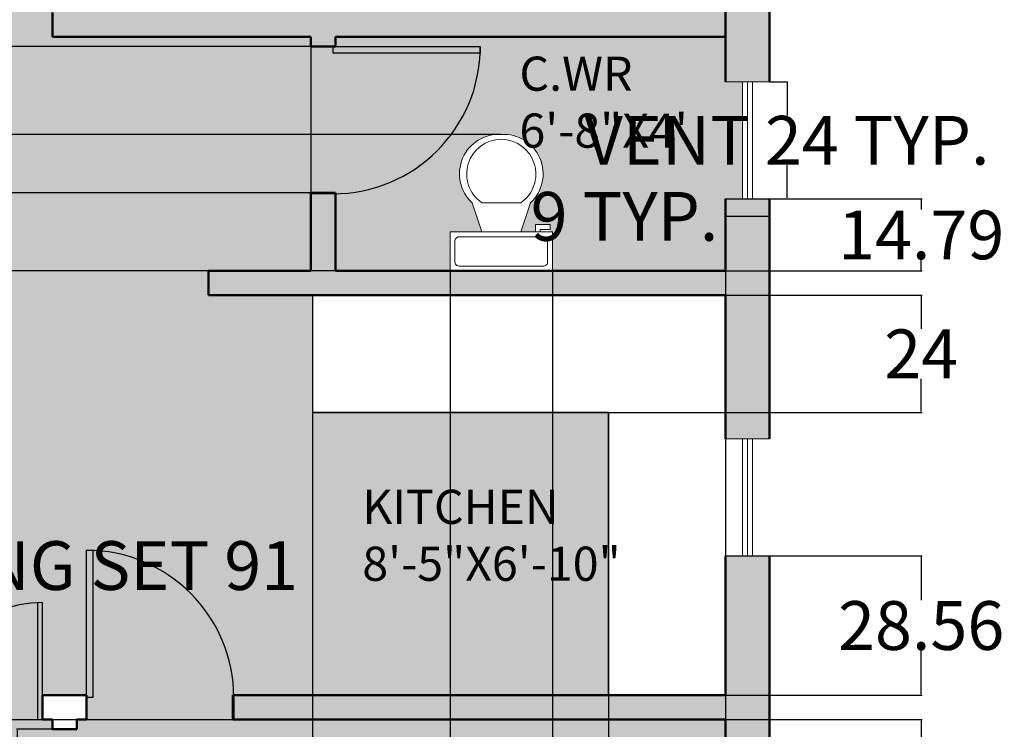
# Model space of a CAD drawing. Units: inches. Extents: x 77 to 548, y 631 to 1307.
# Tile 3 of 4: x 287 to 489, y 856 to 1001. Entities that reach past the tile are written whole.
import ezdxf

# ---------------------------------------------------------------- set-up
doc = ezdxf.new("R2010")
doc.units = ezdxf.units.IN
doc.header["$MEASUREMENT"] = 0
for name, color, linetype, lineweight in [('A-ANNO-DIMS', 2, 'Continuous', 18), ('A-AREA-IDEN', 7, 'Continuous', 18), ('A-FLOR-CASE', 8, 'Continuous', 25), ('A-FLOR-FIXT', 8, 'Continuous', 18), ('A-WALL', 7, 'Continuous', 50), ('DOORS', 4, 'Continuous', 25), ('VENT', 1, 'Continuous', 18)]:
    doc.layers.add(name, color=color, linetype=linetype, lineweight=lineweight)
doc.layers.add('A-FLOR-PATT', color=254, linetype='Continuous', lineweight=13, true_color=0xd7ebd2)
doc.layers.add('A-WALL-PATT', color=252, linetype='Continuous', lineweight=13, true_color=0x939598)
doc.styles.get("Standard").update_dxf_attribs({"font": 'arial.ttf'})
doc.dimstyles.get("Standard").update_dxf_attribs({"dimtxt": 10, "dimasz": 0.18, "dimexe": 0.18, "dimexo": 0.0625, "dimgap": 0.09, "dimtad": 0, "dimtih": 1, "dimtoh": 1, "dimdec": 0, "dimzin": 0, "dimdsep": 46, "dimlunit": 3, "dimtxsty": 'Standard', "dimcen": 0.09, "dimadec": 0, "dimazin": 0, "dimtfac": 1, "dimtdec": 0, "dimtofl": 0, "dimtmove": 0, "dimatfit": 3, "dimfxl": 1, "dimtolj": 1, "dimtzin": 0, "dimarcsym": 0})

# ---------------------------------------------------------------- blocks, each defined once
blk = doc.blocks.new('*U5')
for p, q in [((0, 0), (0, -6)), ((40, 0), (40, -6))]:
    blk.add_line(p, q)
blk.add_lwpolyline([(0, 0), (0, 40), (1.75, 40), (1.75, 0)], close=True)
blk.add_arc((0, 0), 40, 0, 90)
blk = doc.blocks.new('*U8')
for p, q in [((9.5, -6), (9.5, -2)), ((-8, -8.5), (-8, -8)), ((-7, -8), (-7, -9.5)), ((-4, -8), (-6, -14)), ((4, -8), (6, -14)), ((-10, -8.5), (-8, -8.5)), ((-10, -9.5), (-10, -8.5)), ((-7, -9.5), (-10, -9.5)), ((4, -14), (-4, -14))]:
    blk.add_line(p, q)
blk.add_lwpolyline([(10.5, -8), (10.5, 0), (-10.5, 0), (-10.5, -8)], close=True)
for points in [[(-9.5, -2), (-9.5, -6)], [(8.5, -1), (-8.5, -1)], [(-8.5, -7), (8.5, -7)]]:
    blk.add_lwpolyline(points)
for centre, radius, start, end in [((-8.625, -1.875), 0.8839, 81.8699, 188.1301), ((8.625, -1.875), 0.8839, 351.8699, 98.1301), ((-8.625, -6.125), 0.8839, 171.869898, 278.1301), ((8.625, -6.125), 0.8839, 261.8699, 8.1301), ((-0.4772, -19.9188), 8.0953, 133.01722, 273.38), ((0.0374, -19.8731), 7.127, 124.50543, 269.7), ((-0.0373, -19.8731), 7.127, 270.3, 55.4946), ((0.4773, -19.9188), 8.0953, 266.62, 46.9828)]:
    blk.add_arc(centre, radius, start, end)
blk = doc.blocks.new('VENT-LIGHT-24')
for p, q in [((9, 24), (0, 24)), ((3.5, 24), (3.5, 0)), ((4.5, 24), (4.5, 0)), ((5.5, 24), (5.5, 0)), ((9, 0), (0, 0))]:
    blk.add_line(p, q)
blk = doc.blocks.new('DOOR-DOUBLE-48')
for p, q in [((0, 0), (0, 24)), ((1, 0), (1, 23.98)), ((47, 0), (47, 23.98)), ((48, 0), (48, 24)), ((0, 0), (1, 0)), ((47, 0), (48, 0))]:
    blk.add_line(p, q)
for centre, start, end in [((0, 0), 0, 90), ((48, 0), 90, 180)]:
    blk.add_arc(centre, 24, start, end)
blk = doc.blocks.new('*D20')
at = {"layer": 'A-ANNO-DIMS', "color": 0, "lineweight": -2, "transparency": 16777216}
for p, q in [((440.73, 988.68), (444.44, 988.68)), ((444.26, 988.5), (444.26, 981.79)), ((444.26, 964.86), (444.26, 971.56)), ((440.73, 964.68), (444.44, 964.68))]:
    blk.add_line(p, q, dxfattribs=at)
at = {"layer": 'A-ANNO-DIMS', "color": 0, "transparency": 16777216}
for points in [[(444.23, 988.5), (444.29, 988.5), (444.26, 988.68)], [(444.23, 964.86), (444.29, 964.86), (444.26, 964.68)]]:
    blk.add_solid(points, dxfattribs=at)
at = {"layer": 'Defpoints', "color": 0, "transparency": 16777216}
for p in [(440.66, 988.68), (440.66, 964.68), (444.26, 964.68)]:
    blk.add_point(p, dxfattribs=at)
at = {"layer": 'A-ANNO-DIMS', "color": 0, "transparency": 16777216, "insert": (444.26, 976.68), "char_height": 10, "attachment_point": 5}
blk.add_mtext('\\A1;VENT 24 TYP.', dxfattribs=at)
blk = doc.blocks.new('*D21')
at = {"layer": 'A-ANNO-DIMS', "color": 0, "lineweight": -2, "transparency": 16777216}
for p, q in [((431.66, 964.62), (431.66, 960.9)), ((440.66, 964.62), (440.66, 960.9)), ((431.66, 961.08), (431.48, 961.08)), ((440.48, 961.08), (431.84, 961.08))]:
    blk.add_line(p, q, dxfattribs=at)
at = {"layer": 'A-ANNO-DIMS', "color": 0, "transparency": 16777216}
for points in [[(431.84, 961.11), (431.84, 961.05), (431.66, 961.08)], [(440.48, 961.11), (440.48, 961.05), (440.66, 961.08)]]:
    blk.add_solid(points, dxfattribs=at)
at = {"layer": 'Defpoints', "color": 0, "transparency": 16777216}
for p in [(431.66, 964.68), (440.66, 964.68), (431.66, 961.08)]:
    blk.add_point(p, dxfattribs=at)
at = {"layer": 'A-ANNO-DIMS', "color": 0, "transparency": 16777216, "insert": (410.94, 961.08), "char_height": 10, "attachment_point": 5}
blk.add_mtext('\\A1;9 TYP.', dxfattribs=at)
blk = doc.blocks.new('*D26')
at = {"layer": 'A-ANNO-DIMS', "color": 0, "lineweight": -2, "transparency": 16777216}
for p, q in [((293.6, 855.89), (286.28, 855.89)), ((286.46, 855.71), (286.46, 837.15)), ((286.46, 808.07), (286.46, 826.62)), ((293.6, 807.89), (286.28, 807.89))]:
    blk.add_line(p, q, dxfattribs=at)
at = {"layer": 'A-ANNO-DIMS', "color": 0, "transparency": 16777216}
for points in [[(286.43, 855.71), (286.49, 855.71), (286.46, 855.89)], [(286.43, 808.07), (286.49, 808.07), (286.46, 807.89)]]:
    blk.add_solid(points, dxfattribs=at)
at = {"layer": 'Defpoints', "color": 0, "transparency": 16777216}
for p in [(293.66, 855.89), (286.46, 807.89), (293.66, 807.89)]:
    blk.add_point(p, dxfattribs=at)
at = {"layer": 'A-ANNO-DIMS', "color": 0, "transparency": 16777216, "insert": (286.46, 831.89), "char_height": 10, "attachment_point": 5}
blk.add_mtext('\\A1;DOUBLE DOOR 48 TYP.', dxfattribs=at)
blk = doc.blocks.new('*D36')
at = {"layer": 'A-ANNO-DIMS', "color": 0, "lineweight": -2, "transparency": 16777216}
for p, q in [((158.85, 903.05), (158.85, 889.28)), ((249.85, 903.05), (249.85, 889.28)), ((159.03, 889.46), (249.67, 889.46)), ((249.85, 889.46), (250.03, 889.46))]:
    blk.add_line(p, q, dxfattribs=at)
at = {"layer": 'A-ANNO-DIMS', "color": 0, "transparency": 16777216}
for points in [[(159.03, 889.49), (159.03, 889.43), (158.85, 889.46)], [(249.67, 889.49), (249.67, 889.43), (249.85, 889.46)]]:
    blk.add_solid(points, dxfattribs=at)
at = {"layer": 'Defpoints', "color": 0, "transparency": 16777216}
for p in [(158.85, 903.11), (249.85, 903.11), (249.85, 889.46)]:
    blk.add_point(p, dxfattribs=at)
at = {"layer": 'A-ANNO-DIMS', "color": 0, "transparency": 16777216, "insert": (297.98, 889.46), "char_height": 10, "attachment_point": 5}
blk.add_mtext('\\A1;DINING SET 91', dxfattribs=at)
blk = doc.blocks.new('*D48')
at = {"layer": 'A-ANNO-DIMS', "color": 0, "lineweight": -2, "transparency": 16777216}
for p, q in [((431.73, 891.45), (471.94, 891.45)), ((471.76, 891.27), (471.76, 882.36)), ((471.76, 863.07), (471.76, 871.97)), ((431.73, 862.89), (471.94, 862.89))]:
    blk.add_line(p, q, dxfattribs=at)
at = {"layer": 'A-ANNO-DIMS', "color": 0, "transparency": 16777216}
for points in [[(471.73, 891.27), (471.79, 891.27), (471.76, 891.45)], [(471.73, 863.07), (471.79, 863.07), (471.76, 862.89)]]:
    blk.add_solid(points, dxfattribs=at)
at = {"layer": 'Defpoints', "color": 0, "transparency": 16777216}
for p in [(431.66, 891.45), (471.76, 891.45), (431.66, 862.89)]:
    blk.add_point(p, dxfattribs=at)
at = {"layer": 'A-ANNO-DIMS', "color": 0, "transparency": 16777216, "insert": (471.76, 877.17), "char_height": 10, "attachment_point": 5}
blk.add_mtext('\\A1;28.56', dxfattribs=at)
blk = doc.blocks.new('*D49')
at = {"layer": 'A-ANNO-DIMS', "color": 0, "lineweight": -2, "transparency": 16777216}
for p, q in [((431.73, 964.68), (471.94, 964.68)), ((471.76, 964.5), (471.76, 962.48)), ((471.76, 950.07), (471.76, 952.09)), ((431.73, 949.89), (471.94, 949.89))]:
    blk.add_line(p, q, dxfattribs=at)
at = {"layer": 'A-ANNO-DIMS', "color": 0, "transparency": 16777216}
for points in [[(471.73, 964.5), (471.79, 964.5), (471.76, 964.68)], [(471.73, 950.07), (471.79, 950.07), (471.76, 949.89)]]:
    blk.add_solid(points, dxfattribs=at)
at = {"layer": 'Defpoints', "color": 0, "transparency": 16777216}
for p in [(431.66, 964.68), (471.76, 964.68), (431.66, 949.89)]:
    blk.add_point(p, dxfattribs=at)
at = {"layer": 'A-ANNO-DIMS', "color": 0, "transparency": 16777216, "insert": (471.76, 957.28), "char_height": 10, "attachment_point": 5}
blk.add_mtext('\\A1;14.79', dxfattribs=at)
blk = doc.blocks.new('*D54')
at = {"layer": 'A-ANNO-DIMS', "color": 0, "lineweight": -2, "transparency": 16777216}
for p, q in [((351.6, 995.89), (109.38, 995.89)), ((109.56, 995.71), (109.56, 986.09)), ((109.56, 966.07), (109.56, 975.69)), ((351.6, 965.89), (109.38, 965.89))]:
    blk.add_line(p, q, dxfattribs=at)
at = {"layer": 'A-ANNO-DIMS', "color": 0, "transparency": 16777216}
for points in [[(109.53, 995.71), (109.59, 995.71), (109.56, 995.89)], [(109.53, 966.07), (109.59, 966.07), (109.56, 965.89)]]:
    blk.add_solid(points, dxfattribs=at)
at = {"layer": 'Defpoints', "color": 0, "transparency": 16777216}
for p in [(109.56, 995.89), (351.66, 995.89), (351.66, 965.89)]:
    blk.add_point(p, dxfattribs=at)
at = {"layer": 'A-ANNO-DIMS', "color": 0, "transparency": 16777216, "insert": (109.56, 980.89), "char_height": 10, "attachment_point": 5}
blk.add_mtext('\\A1;30', dxfattribs=at)
blk = doc.blocks.new('*D55')
at = {"layer": 'A-ANNO-DIMS', "color": 0, "lineweight": -2, "transparency": 16777216}
for p, q in [((325.73, 944.89), (471.94, 944.89)), ((471.76, 944.71), (471.76, 938)), ((471.76, 921.07), (471.76, 927.78)), ((347.05, 920.89), (471.94, 920.89))]:
    blk.add_line(p, q, dxfattribs=at)
at = {"layer": 'A-ANNO-DIMS', "color": 0, "transparency": 16777216}
for points in [[(471.73, 944.71), (471.79, 944.71), (471.76, 944.89)], [(471.73, 921.07), (471.79, 921.07), (471.76, 920.89)]]:
    blk.add_solid(points, dxfattribs=at)
at = {"layer": 'Defpoints', "color": 0, "transparency": 16777216}
for p in [(325.66, 944.89), (471.76, 944.89), (346.99, 920.89)]:
    blk.add_point(p, dxfattribs=at)
at = {"layer": 'A-ANNO-DIMS', "color": 0, "transparency": 16777216, "insert": (471.76, 932.89), "char_height": 10, "attachment_point": 5}
blk.add_mtext('\\A1;24', dxfattribs=at)
blk = doc.blocks.new('*D57')
at = {"layer": 'A-ANNO-DIMS', "color": 0, "lineweight": -2, "transparency": 16777216}
for p, q in [((346.99, 920.83), (346.99, 637.61)), ((407.66, 920.83), (407.66, 637.61)), ((347.17, 637.79), (360.34, 637.79)), ((407.48, 637.79), (394.32, 637.79))]:
    blk.add_line(p, q, dxfattribs=at)
at = {"layer": 'A-ANNO-DIMS', "color": 0, "transparency": 16777216}
for points in [[(347.17, 637.82), (347.17, 637.76), (346.99, 637.79)], [(407.48, 637.82), (407.48, 637.76), (407.66, 637.79)]]:
    blk.add_solid(points, dxfattribs=at)
at = {"layer": 'Defpoints', "color": 0, "transparency": 16777216}
for p in [(346.99, 920.89), (407.66, 920.89), (407.66, 637.79)]:
    blk.add_point(p, dxfattribs=at)
at = {"layer": 'A-ANNO-DIMS', "color": 0, "transparency": 16777216, "insert": (377.33, 637.79), "char_height": 10, "attachment_point": 5}
blk.add_mtext('\\A1;60.67', dxfattribs=at)
blk = doc.blocks.new('*D58')
at = {"layer": 'A-ANNO-DIMS', "color": 0, "lineweight": -2, "transparency": 16777216}
for p, q in [((375.18, 949.83), (375.18, 637.61)), ((396.18, 949.83), (396.18, 637.61)), ((375.36, 637.79), (379.31, 637.79)), ((396, 637.79), (392.05, 637.79))]:
    blk.add_line(p, q, dxfattribs=at)
at = {"layer": 'A-ANNO-DIMS', "color": 0, "transparency": 16777216}
for points in [[(375.36, 637.82), (375.36, 637.76), (375.18, 637.79)], [(396, 637.82), (396, 637.76), (396.18, 637.79)]]:
    blk.add_solid(points, dxfattribs=at)
at = {"layer": 'Defpoints', "color": 0, "transparency": 16777216}
for p in [(375.18, 949.89), (396.18, 949.89), (396.18, 637.79)]:
    blk.add_point(p, dxfattribs=at)
at = {"layer": 'A-ANNO-DIMS', "color": 0, "transparency": 16777216, "insert": (385.68, 637.79), "char_height": 10, "attachment_point": 5}
blk.add_mtext('\\A1;21', dxfattribs=at)
blk = doc.blocks.new('*D59')
at = {"layer": 'A-ANNO-DIMS', "color": 0, "lineweight": -2, "transparency": 16777216}
for p, q in [((385.62, 977.89), (109.38, 977.89)), ((109.56, 977.71), (109.56, 969.08)), ((109.56, 950.07), (109.56, 958.69)), ((375.12, 949.89), (109.38, 949.89))]:
    blk.add_line(p, q, dxfattribs=at)
at = {"layer": 'A-ANNO-DIMS', "color": 0, "transparency": 16777216}
for points in [[(109.53, 977.71), (109.59, 977.71), (109.56, 977.89)], [(109.53, 950.07), (109.59, 950.07), (109.56, 949.89)]]:
    blk.add_solid(points, dxfattribs=at)
at = {"layer": 'Defpoints', "color": 0, "transparency": 16777216}
for p in [(109.56, 977.89), (385.68, 977.89), (375.18, 949.89)]:
    blk.add_point(p, dxfattribs=at)
at = {"layer": 'A-ANNO-DIMS', "color": 0, "transparency": 16777216, "insert": (109.56, 963.89), "char_height": 10, "attachment_point": 5}
blk.add_mtext('\\A1;28', dxfattribs=at)
blk = doc.blocks.new('*D60')
at = {"layer": 'A-ANNO-DIMS', "color": 0, "lineweight": -2, "transparency": 16777216}
for p, q in [((396.18, 949.83), (396.18, 637.61)), ((431.66, 949.83), (431.66, 637.61)), ((396.36, 637.79), (396.95, 637.79)), ((431.48, 637.79), (430.89, 637.79))]:
    blk.add_line(p, q, dxfattribs=at)
at = {"layer": 'A-ANNO-DIMS', "color": 0, "transparency": 16777216}
for points in [[(396.36, 637.82), (396.36, 637.76), (396.18, 637.79)], [(431.48, 637.82), (431.48, 637.76), (431.66, 637.79)]]:
    blk.add_solid(points, dxfattribs=at)
at = {"layer": 'Defpoints', "color": 0, "transparency": 16777216}
for p in [(396.18, 949.89), (431.66, 949.89), (431.66, 637.79)]:
    blk.add_point(p, dxfattribs=at)
at = {"layer": 'A-ANNO-DIMS', "color": 0, "transparency": 16777216, "insert": (413.92, 637.79), "char_height": 10, "attachment_point": 5}
blk.add_mtext('\\A1;35.48', dxfattribs=at)
blk = doc.blocks.new('*D62')
at = {"layer": 'A-ANNO-DIMS', "color": 0, "lineweight": -2, "transparency": 16777216}
for p, q in [((243.73, 857.89), (471.94, 857.89)), ((471.76, 857.71), (471.76, 837.98)), ((471.76, 807.86), (471.76, 827.59)), ((243.73, 807.68), (471.94, 807.68))]:
    blk.add_line(p, q, dxfattribs=at)
at = {"layer": 'A-ANNO-DIMS', "color": 0, "transparency": 16777216}
for points in [[(471.73, 857.71), (471.79, 857.71), (471.76, 857.89)], [(471.73, 807.86), (471.79, 807.86), (471.76, 807.68)]]:
    blk.add_solid(points, dxfattribs=at)
at = {"layer": 'Defpoints', "color": 0, "transparency": 16777216}
for p in [(243.66, 857.89), (471.76, 857.89), (243.66, 807.68)]:
    blk.add_point(p, dxfattribs=at)
at = {"layer": 'A-ANNO-DIMS', "color": 0, "transparency": 16777216, "insert": (471.76, 832.79), "char_height": 10, "attachment_point": 5}
blk.add_mtext('\\A1;50.2', dxfattribs=at)
blk = doc.blocks.new('*D68')
at = {"layer": 'A-ANNO-DIMS', "color": 0, "lineweight": -2, "transparency": 16777216}
for p, q in [((293.57, 855.89), (293.75, 855.89)), ((293.66, 855.8), (293.66, 855.98)), ((320.82, 828.74), (310.76, 838.79)), ((321, 828.74), (320.82, 828.74))]:
    blk.add_line(p, q, dxfattribs=at)
at = {"layer": 'A-ANNO-DIMS', "color": 0, "transparency": 16777216}
blk.add_solid([(310.78, 838.81), (310.74, 838.77), (310.63, 838.92)], dxfattribs=at)
at = {"layer": 'Defpoints', "color": 0, "transparency": 16777216}
for p in [(293.66, 855.89), (310.63, 838.92)]:
    blk.add_point(p, dxfattribs=at)
at = {"layer": 'A-ANNO-DIMS', "color": 0, "transparency": 16777216, "insert": (343.96, 828.74), "char_height": 10, "attachment_point": 5}
blk.add_mtext('\\A1;4X R24', dxfattribs=at)

msp = doc.modelspace()

# ---------------------------------------------------------------- hatches: boundary and pattern name
at = {"layer": 'A-FLOR-PATT'}
h = msp.add_hatch(color=256, dxfattribs=at)
h.dxf.hatch_style = 1
h.paths.add_polyline_path([(293.663, 1206.888), (291.663, 1206.888), (291.663, 1211.888), (293.663, 1211.888), (293.663, 1259.888), (149.663, 1259.888), (149.663, 1211.888), (257.663, 1211.888), (257.663, 1206.888), (245.663, 1206.888), (245.663, 1204.888), (245.663, 1174.888), (245.663, 1153.888), (149.663, 1153.888), (149.663, 1047.888), (255.663, 1047.888), (255.663, 1042.888), (149.663, 1042.888), (149.663, 988.888), (146.163, 988.888), (146.163, 916.888), (149.663, 916.888), (149.663, 862.888), (243.663, 862.888), (243.663, 857.888), (243.663, 807.683), (293.663, 807.888), (298.663, 807.888), (298.663, 677.888), (431.663, 677.888), (431.663, 702.459), (435.163, 702.459), (435.163, 774.459), (431.663, 774.459), (431.663, 857.888), (330.663, 857.888), (330.663, 862.888), (325.663, 944.888), (325.663, 949.888), (346.663, 949.888), (346.663, 965.888), (346.663, 995.888), (346.663, 997.888), (293.663, 997.888), (293.663, 1002.888), (293.663, 1004.888), (298.663, 1004.888), (298.663, 1002.888), (431.663, 1002.888), (431.663, 1095.888), (431.663, 1100.888), (431.663, 1147.888), (342.663, 1147.888), (342.663, 1174.888), (342.663, 1204.888), (342.663, 1206.888), (334.663, 1206.888), (334.663, 1211.888), (431.663, 1211.888), (431.663, 1259.888), (298.663, 1259.888), (298.663, 1211.888), (300.663, 1211.888), (300.663, 1206.888), (298.663, 1206.888), (298.663, 1042.888), (298.663, 1040.888), (293.663, 1040.888), (291.663, 1040.888), (291.663, 1047.888), (293.663, 1047.888)])
h.paths.add_polyline_path([(291.663, 862.888), (293.663, 862.888), (298.663, 862.888), (300.663, 862.888), (300.663, 857.888), (298.663, 857.888), (298.663, 855.888), (293.663, 855.888), (293.663, 857.888), (291.663, 857.888)], flags=16)
h.paths.add_polyline_path([(407.663, 920.888), (346.988, 920.888), (346.988, 944.888), (325.663, 944.888), (330.663, 862.888), (407.663, 862.888)], flags=17)
h.paths.add_polyline_path([(435.163, 988.679), (431.663, 988.679), (431.663, 997.888), (351.663, 997.888), (351.663, 995.888), (346.663, 995.888), (346.663, 965.888), (351.663, 965.888), (351.663, 949.888), (375.18, 949.888), (375.18, 957.888), (381.68, 957.888), (379.68, 963.887, -0.7025712), (385.68, 977.887, -0.7025621), (391.68, 963.888), (389.68, 957.888), (392.68, 957.888), (392.68, 959.388), (395.68, 959.388), (395.68, 957.888), (396.18, 957.888), (396.18, 949.888), (431.663, 949.888), (431.663, 964.679), (435.163, 964.679)])
h.paths.add_polyline_path([(431.663, 1206.888), (347.663, 1206.888), (347.663, 1204.888), (342.663, 1204.888), (342.663, 1174.888), (347.663, 1174.888), (347.663, 1167.048), (372.327, 1167.048), (372.327, 1152.888), (374.776, 1152.888), (374.776, 1160.888), (381.276, 1160.888), (379.276, 1166.887, -0.7025712), (385.276, 1180.887, -0.7025621), (391.276, 1166.888), (389.276, 1160.888), (392.276, 1160.888), (392.276, 1162.388), (395.276, 1162.388), (395.276, 1160.888), (395.776, 1160.888), (395.776, 1152.888), (431.663, 1152.888), (431.663, 1170.888), (435.163, 1170.888), (435.163, 1194.888), (431.663, 1194.888)])
h.paths.add_polyline_path([(245.663, 1204.888), (240.663, 1204.888), (240.663, 1206.888), (149.663, 1206.888), (149.663, 1194.888), (146.163, 1194.888), (146.163, 1170.888), (149.663, 1170.888), (149.663, 1158.888), (188.741, 1158.888), (188.741, 1166.888), (195.241, 1166.888), (193.241, 1172.887, -0.7025712), (199.241, 1186.887, -0.7025621), (205.241, 1172.888), (203.241, 1166.888), (206.241, 1166.888), (206.241, 1168.388), (209.241, 1168.388), (209.241, 1166.888), (209.741, 1166.888), (209.741, 1158.888), (215.999, 1158.888), (215.999, 1173.048), (240.663, 1173.048), (240.663, 1174.888), (245.663, 1174.888)], flags=17)
at = {"layer": 'A-WALL-PATT'}
h = msp.add_hatch(color=256, dxfattribs=at)
h.dxf.hatch_style = 1
h.paths.add_polyline_path([(149.663, 1042.888), (149.663, 1170.888), (140.663, 1170.888), (140.663, 988.888), (149.663, 988.888)])
h.paths.add_polyline_path([(149.663, 1259.888), (431.663, 1259.888), (431.663, 1194.888), (440.663, 1194.888), (440.663, 1268.888), (140.663, 1268.888), (140.663, 1194.888), (149.663, 1194.888), (149.663, 1206.888)])
h.paths.add_polyline_path([(298.663, 1259.888), (293.663, 1259.888), (293.663, 1211.888), (291.663, 1211.888), (291.663, 1206.888), (293.663, 1206.888), (293.663, 1047.888), (291.663, 1047.888), (291.663, 1040.888), (293.663, 1040.888), (298.663, 1040.888), (298.663, 1095.888), (298.663, 1206.888), (300.663, 1206.888), (300.663, 1211.888), (298.663, 1211.888)])
h.paths.add_polyline_path([(257.663, 1211.888), (149.663, 1211.888), (149.663, 1206.888), (240.663, 1206.888), (240.663, 1204.888), (241.135, 1204.888), (245.663, 1204.888), (245.663, 1206.888), (257.663, 1206.888)], flags=17)
h.paths.add_polyline_path([(431.663, 1211.888), (334.663, 1211.888), (334.663, 1206.888), (342.663, 1206.888), (342.663, 1204.888), (347.191, 1204.888), (347.663, 1204.888), (347.663, 1206.888), (431.663, 1206.888)], flags=17)
h.paths.add_polyline_path([(440.663, 1170.888), (431.663, 1170.888), (431.663, 1100.888), (431.663, 1047.888), (431.663, 988.679), (440.663, 988.679)])
h.paths.add_polyline_path([(431.663, 1002.888), (298.663, 1002.888), (298.663, 1004.888), (293.663, 1004.888), (293.663, 1002.888), (293.663, 997.888), (346.663, 997.888), (346.663, 995.888), (351.663, 995.888), (351.663, 997.888), (431.663, 997.888)])
h.paths.add_polyline_path([(440.663, 964.679), (431.663, 964.679), (431.663, 949.888), (351.663, 949.888), (351.663, 965.888), (346.663, 965.888), (346.663, 949.888), (325.663, 949.888), (325.663, 944.888), (431.663, 944.888), (431.663, 915.45), (440.663, 915.45)])
h.paths.add_polyline_path([(440.663, 891.45), (431.663, 891.45), (431.663, 862.888), (330.663, 862.888), (330.663, 857.888), (431.663, 857.888), (431.663, 774.459), (440.663, 774.459)], flags=17)
h.paths.add_polyline_path([(440.663, 702.459), (431.663, 702.459), (431.663, 677.888), (149.663, 677.888), (149.663, 916.888), (140.663, 916.888), (140.663, 668.888), (440.663, 668.888)])
h.paths.add_polyline_path([(293.663, 807.888), (243.663, 807.683), (243.663, 857.888), (233.663, 857.888), (233.663, 807.683), (233.663, 797.642), (243.704, 797.683), (293.663, 797.887)], flags=17)
h.paths.add_polyline_path([(243.663, 862.888), (149.663, 862.888), (149.663, 857.888), (243.663, 857.888)], flags=17)

# ---------------------------------------------------------------- linework, layer by layer
at = {"layer": 'A-FLOR-CASE'}
for p, q in [((346.988, 944.888), (346.988, 920.888)), ((407.663, 920.888), (346.988, 920.888)), ((407.663, 862.888), (407.663, 920.888))]:
    msp.add_line(p, q, dxfattribs=at)
at = {"layer": 'A-WALL'}
for p, q in [((440.663, 988.679), (440.663, 1170.888)), ((431.663, 988.679), (431.663, 1095.888)), ((293.663, 997.888), (293.663, 1002.888)), ((346.663, 997.888), (293.663, 997.888)), ((346.663, 997.888), (346.663, 995.888)), ((431.663, 997.888), (351.663, 997.888)), ((351.663, 995.888), (351.663, 997.888)), ((346.663, 995.888), (351.663, 995.888)), ((346.663, 949.888), (346.663, 965.888)), ((351.663, 965.888), (346.663, 965.888)), ((351.663, 949.888), (351.663, 965.888)), ((431.663, 949.888), (431.663, 964.679)), ((440.663, 915.45), (440.663, 964.679)), ((346.663, 949.888), (325.663, 949.888)), ((325.663, 944.888), (325.663, 949.888)), ((431.663, 949.888), (351.663, 949.888)), ((431.663, 944.888), (325.663, 944.888)), ((431.663, 915.45), (431.663, 944.888)), ((431.663, 862.888), (431.663, 891.45)), ((440.663, 774.459), (440.663, 891.45)), ((291.663, 857.888), (291.663, 862.888)), ((291.663, 862.888), (293.663, 862.888)), ((293.663, 862.888), (298.663, 862.888)), ((298.663, 862.888), (300.663, 862.888)), ((300.663, 862.888), (300.663, 857.888)), ((330.663, 862.888), (431.663, 862.888)), ((330.663, 857.888), (330.663, 862.888)), ((293.663, 857.888), (291.663, 857.888)), ((293.663, 857.888), (291.663, 857.888)), ((293.663, 857.888), (293.663, 855.888)), ((300.663, 857.888), (298.663, 857.888)), ((298.663, 855.888), (298.663, 857.888)), ((300.663, 857.888), (300.663, 857.888)), ((330.663, 857.888), (431.663, 857.888)), ((431.663, 774.459), (431.663, 857.888)), ((293.663, 855.888), (298.663, 855.888))]:
    msp.add_line(p, q, dxfattribs=at)
at = {"layer": 'DOORS'}
msp.add_line((346.663, 995.888), (346.663, 965.888), dxfattribs=at)

# ---------------------------------------------------------------- block references
at = {"layer": 'A-FLOR-FIXT', "rotation": 180}
msp.add_blockref('*U8', (385.68, 949.888), dxfattribs=at)
at = {"layer": 'DOORS', "xscale": 0.7547077719127327, "yscale": 0.7547077719127327, "zscale": 0.7547077719127327, "rotation": 270}
msp.add_blockref('*U5', (351.191, 995.888), dxfattribs=at)
at = {"layer": 'DOORS', "xscale": 0.7547077719127327, "yscale": 0.7547077719127327, "zscale": 0.7547077719127327}
msp.add_blockref('*U5', (300.663, 862.416), dxfattribs=at)
at = {"layer": 'DOORS'}
msp.add_blockref('DOOR-DOUBLE-48', (243.663, 857.888), dxfattribs=at)
at = {"layer": 'VENT', "rotation": 180}
for p in [(440.663, 988.678), (440.663, 915.449)]:
    msp.add_blockref('VENT-LIGHT-24', p, dxfattribs=at)

# ---------------------------------------------------------------- texts
at = {"layer": 'A-AREA-IDEN', "char_height": 5, "attachment_point": 1}
for s, insert in [('{\\H1.4x;C.WR\\P6\'-8"X4\'}', (389.399, 993.842)), ('{\\H1.4x;KITCHEN\\P8\'-5"X6\'-10"}', (357.19, 905.012))]:
    msp.add_mtext_dynamic_manual_height_columns(s, width=19.9597, gutter_width=1, heights=[0], dxfattribs=dict(at, insert=insert))

# ---------------------------------------------------------------- dimensions: what is measured, and where the dimension line sits
at = {"layer": 'A-ANNO-DIMS'}
for base, p1, p2, angle, text, picture, middle in [((444.263, 964.679), (440.663, 988.679), (440.663, 964.679), 270, 'VENT <> TYP.', '*D20', (444.263, 976.679)), ((431.663, 961.079), (440.663, 964.679), (431.663, 964.679), 180, '<> TYP.', '*D21', (410.939, 961.079)), ((286.463, 807.888), (293.663, 855.888), (293.663, 807.888), 270, 'DOUBLE DOOR <> TYP.', '*D26', (286.463, 831.888))]:
    dim = msp.add_linear_dim(base=base, p1=p1, p2=p2, angle=angle, text=text, dimstyle='Standard', override={"dimdec": 0, "dimlfac": 1, "dimrnd": 0, "dimzin": 0, "dimdsep": 46, "dimlunit": 2}, dxfattribs=at)
    dim.commit()
    dim.dimension.update_dxf_attribs({"geometry": picture, "text_midpoint": middle})
for base, p1, p2, override, picture, middle in [((109.563, 995.888), (351.663, 965.888), (351.663, 995.888), {"dimdec": 0, "dimlfac": 1, "dimrnd": 0, "dimzin": 0, "dimdsep": 46, "dimlunit": 2}, '*D54', (109.563, 980.888)), ((109.563, 977.887), (375.18, 949.888), (385.68, 977.887), {"dimdec": 0, "dimlfac": 1, "dimrnd": 0, "dimzin": 0, "dimdsep": 46, "dimlunit": 2}, '*D59', (109.563, 963.887)), ((471.763, 964.679), (431.663, 949.888), (431.663, 964.679), {"dimdec": 2, "dimlfac": 1, "dimrnd": 0, "dimzin": 0, "dimdsep": 46, "dimlunit": 2}, '*D49', (471.763, 957.283)), ((471.763, 944.888), (346.988, 920.888), (325.663, 944.888), {"dimdec": 0, "dimlfac": 1, "dimrnd": 0, "dimzin": 0, "dimdsep": 46, "dimlunit": 2}, '*D55', (471.763, 932.888)), ((471.763, 891.45), (431.663, 862.888), (431.663, 891.45), {"dimdec": 2, "dimlfac": 1, "dimrnd": 0, "dimzin": 0, "dimdsep": 46, "dimlunit": 2}, '*D48', (471.763, 877.169)), ((471.763, 857.888), (243.663, 807.683), (243.663, 857.888), {"dimdec": 1, "dimlfac": 1, "dimrnd": 0, "dimzin": 0, "dimdsep": 46, "dimlunit": 2}, '*D62', (471.763, 832.785))]:
    dim = msp.add_linear_dim(base=base, p1=p1, p2=p2, angle=90, dimstyle='Standard', override=override, dxfattribs=at)
    dim.commit()
    dim.dimension.update_dxf_attribs({"geometry": picture, "text_midpoint": middle})
for base, p1, p2, override, picture, middle in [((396.18, 637.788), (375.18, 949.888), (396.18, 949.888), {"dimdec": 0, "dimlfac": 1, "dimrnd": 0, "dimzin": 0, "dimdsep": 46, "dimlunit": 2}, '*D58', (385.68, 637.788)), ((431.663, 637.788), (396.18, 949.888), (431.663, 949.888), {"dimdec": 2, "dimlfac": 1, "dimrnd": 0, "dimzin": 0, "dimdsep": 46, "dimlunit": 2}, '*D60', (413.922, 637.788)), ((407.663, 637.7875), (346.9885, 920.8875), (407.663, 920.8875), {"dimdec": 2, "dimlfac": 1, "dimrnd": 0, "dimzin": 0, "dimdsep": 46, "dimlunit": 2}, '*D57', (377.3257, 637.7875))]:
    dim = msp.add_linear_dim(base=base, p1=p1, p2=p2, dimstyle='Standard', override=override, dxfattribs=at)
    dim.commit()
    dim.dimension.update_dxf_attribs({"geometry": picture, "text_midpoint": middle})
dim = msp.add_linear_dim(base=(249.85, 889.462), p1=(158.85, 903.112), p2=(249.85, 903.112), text='DINING SET <>', dimstyle='Standard', override={"dimdec": 0, "dimlfac": 1, "dimrnd": 0, "dimzin": 0, "dimdsep": 46, "dimlunit": 2}, dxfattribs=at)
dim.commit()
dim.dimension.update_dxf_attribs({"geometry": '*D36', "text_midpoint": (297.981, 889.462)})
dim = msp.add_radius_dim(center=(293.663, 855.888), mpoint=(310.634, 838.917), text='4X <>', dimstyle='Standard', override={"dimdec": 0, "dimlfac": 1, "dimrnd": 0, "dimzin": 0, "dimdsep": 46, "dimlunit": 2}, dxfattribs=at)
dim.commit()
dim.dimension.update_dxf_attribs({"geometry": '*D68', "text_midpoint": (343.958, 828.735), "dimtype": 164})

doc.saveas('drawing.dxf')
